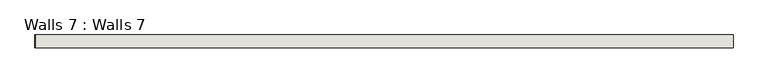
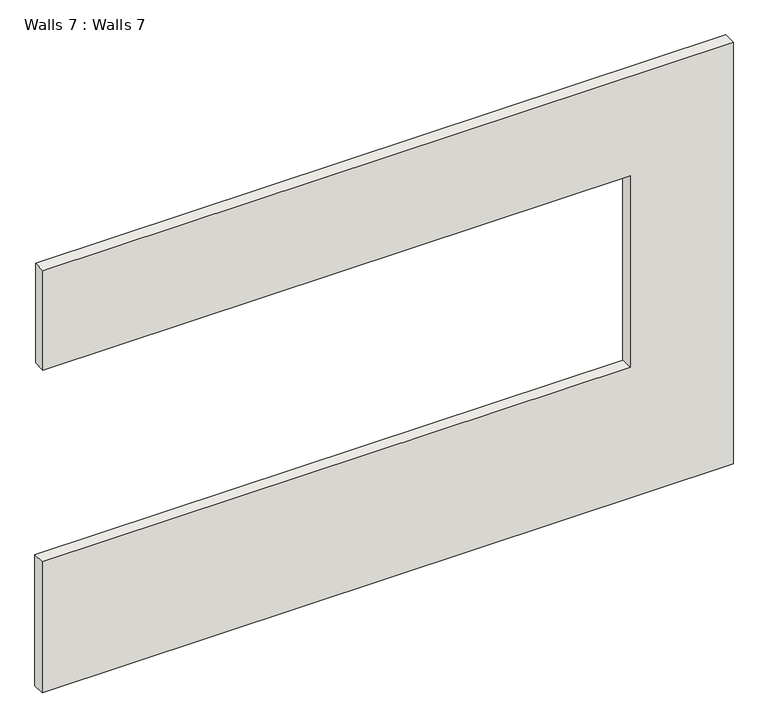
"""IFC4 building model written with IfcOpenShell, lengths in millimetres: wall geometry, Walls 7 : Walls 7."""

from ifc_helpers import new_model, si_unit, frame, origin, place, context, project, spatial, polyline, outline, extrude, source, transform, mapped, element, save


def walls_7_walls_7_28da2d4c(model_context):
    return source(origin(), model_context, "Body", "SweptSolid", [
        extrude(outline(polyline([(18592.8, -1558.2162602), (18592.8, -8965.1585888), (17464.824337, -8965.1585888), (17464.824337, -2663.3436544), (15290.9131351, -2663.3436544), (15290.9131351, -8972.7907061), (13807.224337, -8972.7907061), (13807.224337, -1558.2162602), (18592.8, -1558.2162602)])), frame((0.0, -4123.912388, 0.0), z_axis=(0.0, 1.0, 0.0), x_axis=(0.0, 0.0, 1.0)), (0.0, 0.0, 1.0), 134.6798126),
    ])


if __name__ == "__main__":
    model = new_model("IFC4")
    model_context = context("Model", 3, world=origin())
    ifc_project = project(units=[si_unit("LENGTHUNIT", "METRE", prefix="MILLI")], contexts=[model_context])
    site = spatial("IfcSite", under=ifc_project)
    building = spatial("IfcBuilding", under=site)
    placement = place(None, origin())
    walls_7_walls_7_shape = walls_7_walls_7_28da2d4c(model_context)
    element("IfcWall", 1, ObjectType="Walls 7 : Walls 7", at=placement, inside=building, context=model_context, shape_type="MappedRepresentation", body=[
        mapped(walls_7_walls_7_shape, transform((0.0, 0.0, 0.0), x_axis=(1.0, 0.0, 0.0), y_axis=(0.0, 1.0, 0.0), z_axis=(0.0, 0.0, 1.0))),
    ])
    save(model, "model.ifc")

# Revit data of these elements
# Element 1 (IfcWall, "Walls 7 : Walls 7")
#   Materials on its faces: "Default Wall"
# Materials
#   "Default Wall": colour RGB 128 128 128, transparency 0
